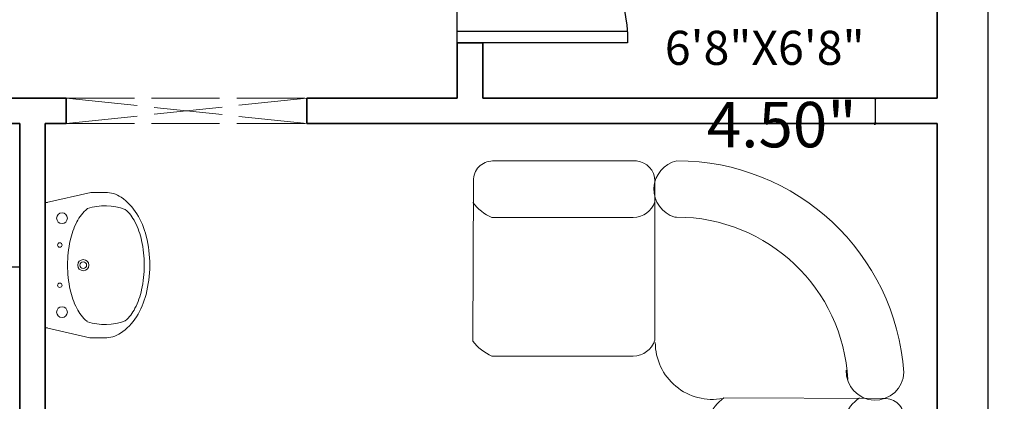
# Model space of a CAD drawing. Units: inches. Extents: x -11 to 443, y 65 to 743.
# Tile 5 of 10: x 162 to 335, y 325 to 392. Entities that reach past the tile are written whole.
import ezdxf

# ---------------------------------------------------------------- set-up
doc = ezdxf.new("R2010")
doc.units = ezdxf.units.IN
doc.header["$MEASUREMENT"] = 0
doc.linetypes.add('ACAD_ISO02W100', pattern=[15, 12, -3])
for name, color, linetype, lineweight in [('A-ANNO-DIMS', 2, 'Continuous', 18), ('A-AREA-IDEN', 2, 'Continuous', 18), ('A-DOOR', 4, 'Continuous', 25), ('A-FLOR-CASE', 8, 'Continuous', 25), ('A-FLOR-FIXT', 8, 'Continuous', 18), ('A-WALL', 7, 'Continuous', 35), ('A-WALL-OVHD', 8, 'ACAD_ISO02W100', 13), ('C-PROP', 3, 'Continuous', 30), ('Furniture', 7, 'Continuous', 15)]:
    doc.layers.add(name, color=color, linetype=linetype, lineweight=lineweight)
doc.styles.get("Standard").update_dxf_attribs({"font": 'italic8.shx'})
doc.dimstyles.get("Standard").update_dxf_attribs({"dimtxt": 8, "dimasz": 0.18, "dimexe": 0.18, "dimexo": 0.0625, "dimgap": 0.09, "dimtad": 0, "dimtih": 1, "dimtoh": 1, "dimzin": 0, "dimdsep": 46, "dimlunit": 3, "dimtxsty": 'Standard', "dimblk": 'CLOSEDBLANK', "dimcen": 0.09, "dimclrd": 6, "dimclre": 5, "dimclrt": 4, "dimadec": 0, "dimazin": 0, "dimtfac": 1, "dimtofl": 0, "dimtmove": 0, "dimatfit": 3, "dimfxl": 1, "dimtolj": 1, "dimtzin": 0, "dimarcsym": 0})

# ---------------------------------------------------------------- blocks, each defined once
blk = doc.blocks.new('_ClosedBlank')
at = {"color": 0, "linetype": 'ByBlock', "lineweight": -2}
for p, q in [((-1, 0.167), (0, 0)), ((-1, 0.167), (-1, -0.167)), ((0, 0), (-1, -0.167))]:
    blk.add_line(p, q, dxfattribs=at)
blk = doc.blocks.new('*D6')
at = {"layer": 'A-ANNO-DIMS', "color": 0, "lineweight": -2, "transparency": 16777216}
for p, q in [((332.27, 706.92), (352.4, 706.92)), ((352.22, 706.74), (352.22, 411.77)), ((352.22, 107.1), (352.22, 402.07)), ((332.27, 106.92), (352.4, 106.92))]:
    blk.add_line(p, q, dxfattribs=at)
at = {"layer": 'Defpoints', "color": 0, "lineweight": 100, "transparency": 16777216}
for p in [(332.21, 706.92), (332.21, 106.92), (352.22, 106.92)]:
    blk.add_point(p, dxfattribs=at)
at = {"layer": 'A-ANNO-DIMS', "color": 0, "lineweight": -2, "transparency": 16777216, "xscale": 0.18, "yscale": 0.18, "zscale": 0.18}
for p, rotation in [((352.22, 706.92), 90), ((352.22, 106.92), 270)]:
    blk.add_blockref('_ClosedBlank', p, dxfattribs=dict(at, rotation=rotation))
at = {"layer": 'A-ANNO-DIMS', "color": 0, "transparency": 16777216, "insert": (352.22, 406.92), "char_height": 8, "attachment_point": 5}
blk.add_mtext("\\A1;50'", dxfattribs=at)
blk = doc.blocks.new('*D8')
at = {"layer": 'A-ANNO-DIMS', "color": 0, "lineweight": -2, "transparency": 16777216}
for p, q in [((312.31, 378.24), (312.31, 374.1)), ((312.37, 378.42), (312.49, 378.42)), ((312.31, 373.74), (312.13, 373.74)), ((312.31, 373.92), (312.31, 373.74)), ((312.37, 373.92), (312.49, 373.92))]:
    blk.add_line(p, q, dxfattribs=at)
at = {"layer": 'Defpoints', "color": 0, "lineweight": 100, "transparency": 16777216}
for p in [(312.31, 378.42), (312.31, 373.92), (312.31, 373.92)]:
    blk.add_point(p, dxfattribs=at)
at = {"layer": 'A-ANNO-DIMS', "color": 0, "lineweight": -2, "transparency": 16777216, "xscale": 0.18, "yscale": 0.18, "zscale": 0.18}
for p, rotation in [((312.31, 378.42), 90), ((312.31, 373.92), 270)]:
    blk.add_blockref('_ClosedBlank', p, dxfattribs=dict(at, rotation=rotation))
at = {"layer": 'A-ANNO-DIMS', "color": 0, "transparency": 16777216, "insert": (295.85, 373.74), "char_height": 8, "attachment_point": 5}
blk.add_mtext('\\A1;4.50"', dxfattribs=at)
blk = doc.blocks.new('DOOR-SWING-30')
for p, q in [((0, 30), (0, 0)), ((2, 29.93), (2, 0)), ((0, 0), (30, 0))]:
    blk.add_line(p, q)
blk.add_arc((0, 0), 30, 0, 90)
blk = doc.blocks.new('SECTIONAL-SEAT')
for p, q in [((30.86, 31.9, -13.5), (2.62, 32.04, -13.5)), ((0, 28.69, -13.5), (0, 3.79, -13.5)), ((23.85, 28.69, -13.5), (23.85, 3.79, -13.5)), ((34.36, 3.2, -13.5), (34.36, 28.55, -13.5)), ((2.77, 0, -13.5), (30.86, 0, -13.5))]:
    blk.add_line(p, q)
for centre, radius, start, end in [((7.52, 25.51, -13.5), 8.17, 126.8838, 157.0502), ((31.38, 25.51, -13.5), 8.17, 126.8838, 157.0502), ((31, 28.55, -13.5), 3.35, 0, 92.4088), ((3.97, 3.79, -13.5), 3.98, 180, 252.2888), ((27.83, 3.79, -13.5), 3.98, 180, 244.0743), ((30.86, 3.51, -13.5), 3.51, 270, 355.0498)]:
    blk.add_arc(centre, radius, start, end)
blk = doc.blocks.new('*D36')
at = {"layer": 'A-ANNO-DIMS', "color": 5, "lineweight": -2, "transparency": 16777216}
for p, q in [((323.27, 625.92), (362.85, 625.92)), ((323.27, 211.92), (362.85, 211.92))]:
    blk.add_line(p, q, dxfattribs=at)
at = {"layer": 'A-ANNO-DIMS', "color": 6, "lineweight": -2, "transparency": 16777216}
for p, q in [((362.67, 625.74), (362.67, 423.77)), ((362.67, 212.1), (362.67, 414.07))]:
    blk.add_line(p, q, dxfattribs=at)
at = {"layer": 'Defpoints', "color": 0, "lineweight": 100, "transparency": 16777216}
for p in [(323.21, 625.92), (362.67, 625.92), (323.21, 211.92)]:
    blk.add_point(p, dxfattribs=at)
at = {"layer": 'A-ANNO-DIMS', "color": 6, "lineweight": -2, "transparency": 16777216, "xscale": 0.18, "yscale": 0.18, "zscale": 0.18}
for p, rotation in [((362.67, 625.92), 90), ((362.67, 211.92), 270)]:
    blk.add_blockref('_ClosedBlank', p, dxfattribs=dict(at, rotation=rotation))
at = {"layer": 'A-ANNO-DIMS', "color": 4, "transparency": 16777216, "insert": (362.67, 418.92), "char_height": 8, "attachment_point": 5}
blk.add_mtext('\\A1;34\'-6"', dxfattribs=at)

msp = doc.modelspace()

# ---------------------------------------------------------------- linework, layer by layer
at = {"layer": 'A-FLOR-CASE'}
for p, q in [((118.155, 348.71), (161.709, 348.71)), ((161.709, 347.562), (161.709, 347.562))]:
    msp.add_line(p, q, dxfattribs=at)
at = {"layer": 'A-FLOR-FIXT'}
for p, q in [((174.228, 361.806), (166.406, 360.006)), ((174.228, 361.806), (176.773, 361.806)), ((166.209, 337.958), (166.209, 360.006)), ((166.209, 360.006), (166.603, 360.006)), ((173.408, 339.227), (173.49, 339.133)), ((173.646, 339.12), (173.519, 339.12)), ((166.603, 337.958), (166.209, 337.958)), ((174.064, 336.161), (166.406, 337.958)), ((174.228, 336.158), (176.773, 336.158))]:
    msp.add_line(p, q, dxfattribs=at)
for centre, radius in [((169.162, 357.25), 0.945), ((168.768, 352.525), 0.394), ((172.902, 348.982), 0.984), ((172.902, 348.982), 0.591), ((168.768, 345.439), 0.394), ((169.162, 340.714), 0.945), ((169.162, 340.714), 0.945), ((169.162, 340.714), 0.945)]:
    msp.add_circle(centre, radius, dxfattribs=at)
for centre, radius, start, end in [((176.753, 356.812), 4.995, 89.76763, 90.96062), ((176.753, 356.812), 4.995, 55.80478, 89.76763), ((174.219, 353.082), 9.504, 31.35734, 55.80478), ((178.631, 353.057), 7.73, 130.39006, 152.8258), ((176.77, 349.514), 9.942, 69.30222, 108.46133), ((175.126, 353.057), 7.73, 27.1742, 48.14439), ((170.194, 350.629), 14.217, 14.0583, 31.35734), ((183.417, 350.6), 13.11, 152.8258, 167.99536), ((170.34, 350.6), 13.11, 12.00464, 27.1742), ((163.825, 349.034), 20.783, 359.76763, 14.0583), ((191.025, 348.982), 20.888, 167.99536, 180), ((162.732, 348.982), 20.888, 0, 12.00464), ((191.025, 348.982), 20.888, 180, 192.00464), ((162.732, 348.982), 20.888, 347.99536, 0), ((163.825, 349.034), 20.783, 345.47696, 359.76763), ((183.417, 347.364), 13.11, 192.00464, 207.1742), ((170.34, 347.364), 13.11, 332.8258, 347.99536), ((170.18, 347.388), 14.217, 328.17791, 345.47696), ((178.631, 344.907), 7.73, 207.1742, 228.62612), ((174.185, 344.902), 9.504, 303.73047, 328.17791), ((175.126, 344.907), 7.73, 311.94987, 332.8258), ((173.519, 339.159), 0.0394, 221.32236, 270), ((176.77, 348.45), 9.942, 251.53867, 290.69778), ((176.689, 341.152), 4.995, 269.76763, 303.73047), ((174.248, 341.152), 4.995, 267.88301, 269.76763)]:
    msp.add_arc(centre, radius, start, end, dxfattribs=at)
at = {"layer": 'A-WALL'}
for p, q in [((323.209, 378.42), (323.209, 457.92)), ((238.709, 378.42), (238.709, 388.17)), ((243.209, 388.17), (238.709, 388.17)), ((243.209, 378.42), (243.209, 388.17)), ((137.709, 378.42), (169.908, 378.42)), ((169.908, 378.42), (169.908, 373.92)), ((212.238, 373.92), (212.238, 378.42)), ((212.238, 378.42), (238.709, 378.42)), ((243.209, 378.42), (323.209, 378.42)), ((91.709, 373.92), (161.709, 373.92)), ((161.709, 275.92), (161.709, 373.92)), ((166.209, 373.92), (169.908, 373.92)), ((166.209, 263.442), (166.209, 373.92)), ((212.238, 373.92), (323.209, 373.92)), ((323.209, 220.92), (323.209, 373.92))]:
    msp.add_line(p, q, dxfattribs=at)
at = {"layer": 'A-WALL-OVHD'}
for p, q in [((169.908, 378.42), (212.238, 378.42)), ((212.238, 378.42), (169.908, 373.92)), ((212.238, 373.92), (169.908, 378.42)), ((169.908, 373.92), (212.238, 373.92))]:
    msp.add_line(p, q, dxfattribs=at)
at = {"layer": 'C-PROP'}
msp.add_lwpolyline([(44.209, 106.92), (332.209, 106.92), (332.209, 706.92), (44.209, 706.92)], close=True, dxfattribs=at)
at = {"layer": 'Furniture'}
for p, q in [((270.307, 367.335, -13.498), (244.963, 367.335, -13.498)), ((241.467, 335.598, -13.498), (241.613, 363.841, -13.498)), ((273.511, 335.744, -13.498), (273.511, 363.841, -13.498)), ((273.511, 360.157, -13.498), (273.511, 360.257, -13.498)), ((244.817, 357.391, -13.498), (269.724, 357.391, -13.498)), ((277.012, 357.441, -13.498), (277.352, 357.441, -13.498)), ((244.817, 332.978, -13.498), (269.724, 332.978, -13.498))]:
    msp.add_line(p, q, dxfattribs=at)
for centre, radius, start, end in [((244.963, 363.982, -13.498), 3.353, 90, 182.40882), ((270.004, 363.841, -13.498), 3.507, 0, 85.04975), ((278.494, 362.361, -13.498), 5.139, 102.42608, 253.23349), ((277.352, 327.293, -13.498), 40.087, 3.98704, 89.94828), ((248.004, 364.916, -13.498), 8.172, 216.8838, 247.05023), ((269.724, 361.366, -13.498), 3.975, 270, 342.28877), ((277.352, 327.293, -13.498), 30.148, 2.91594, 90), ((248.004, 340.503, -13.498), 8.172, 216.8838, 247.05023), ((269.724, 336.953, -13.498), 3.975, 270, 342.28877), ((283.629, 335.376, -13.498), 10.046, 180, 280.60062), ((312.268, 330.277, -13.498), 5.079, 178.01213, 358.01213)]:
    msp.add_arc(centre, radius, start, end, dxfattribs=at)

# ---------------------------------------------------------------- block references
at = {"layer": 'A-DOOR', "extrusion": (0, 0, -1), "zscale": -1, "rotation": 90.00000000000003}
msp.add_blockref('DOOR-SWING-30', (-238.709, 388.169), dxfattribs=at)
at = {"layer": 'Furniture'}
msp.add_blockref('SECTIONAL-SEAT', (283.033, 293.573), dxfattribs=at)

# ---------------------------------------------------------------- texts
at = {"layer": 'A-AREA-IDEN'}
msp.add_text('6\'8"X6\'8"', height=6, dxfattribs=at).set_placement((275.264, 384.271))
at = {"layer": 'A-FLOR-FIXT', "width": 0.8, "flags": 9}
for tag, s in [('XSIZE', '650'), ('YSIZE', '450')]:
    msp.add_attdef(tag, (166.209, 348.982), s, height=0.0197, rotation=90, dxfattribs=at)

# ---------------------------------------------------------------- dimensions: what is measured, and where the dimension line sits
at = {"layer": 'A-ANNO-DIMS'}
for base, p1, p2, override, picture, middle in [((352.221, 106.92), (332.209, 706.92), (332.209, 106.92), {"dimclrd": 0, "dimclre": 0, "dimclrt": 0}, '*D6', (352.221, 406.92)), ((362.669, 625.92), (323.209, 211.92), (323.209, 625.92), {"dimdec": 1, "dimlfac": 1, "dimrnd": 0, "dimzin": 1, "dimdsep": 46, "dimlunit": 4, "dimfrac": 2}, '*D36', (362.669, 418.92)), ((312.307, 373.92), (312.307, 378.42), (312.307, 373.92), {"dimclrd": 0, "dimclre": 0, "dimclrt": 0}, '*D8', (295.846, 373.74))]:
    dim = msp.add_linear_dim(base=base, p1=p1, p2=p2, angle=90, dimstyle='Standard', override=override, dxfattribs=at)
    dim.commit()
    dim.dimension.update_dxf_attribs({"geometry": picture, "text_midpoint": middle})

doc.saveas('drawing.dxf')
